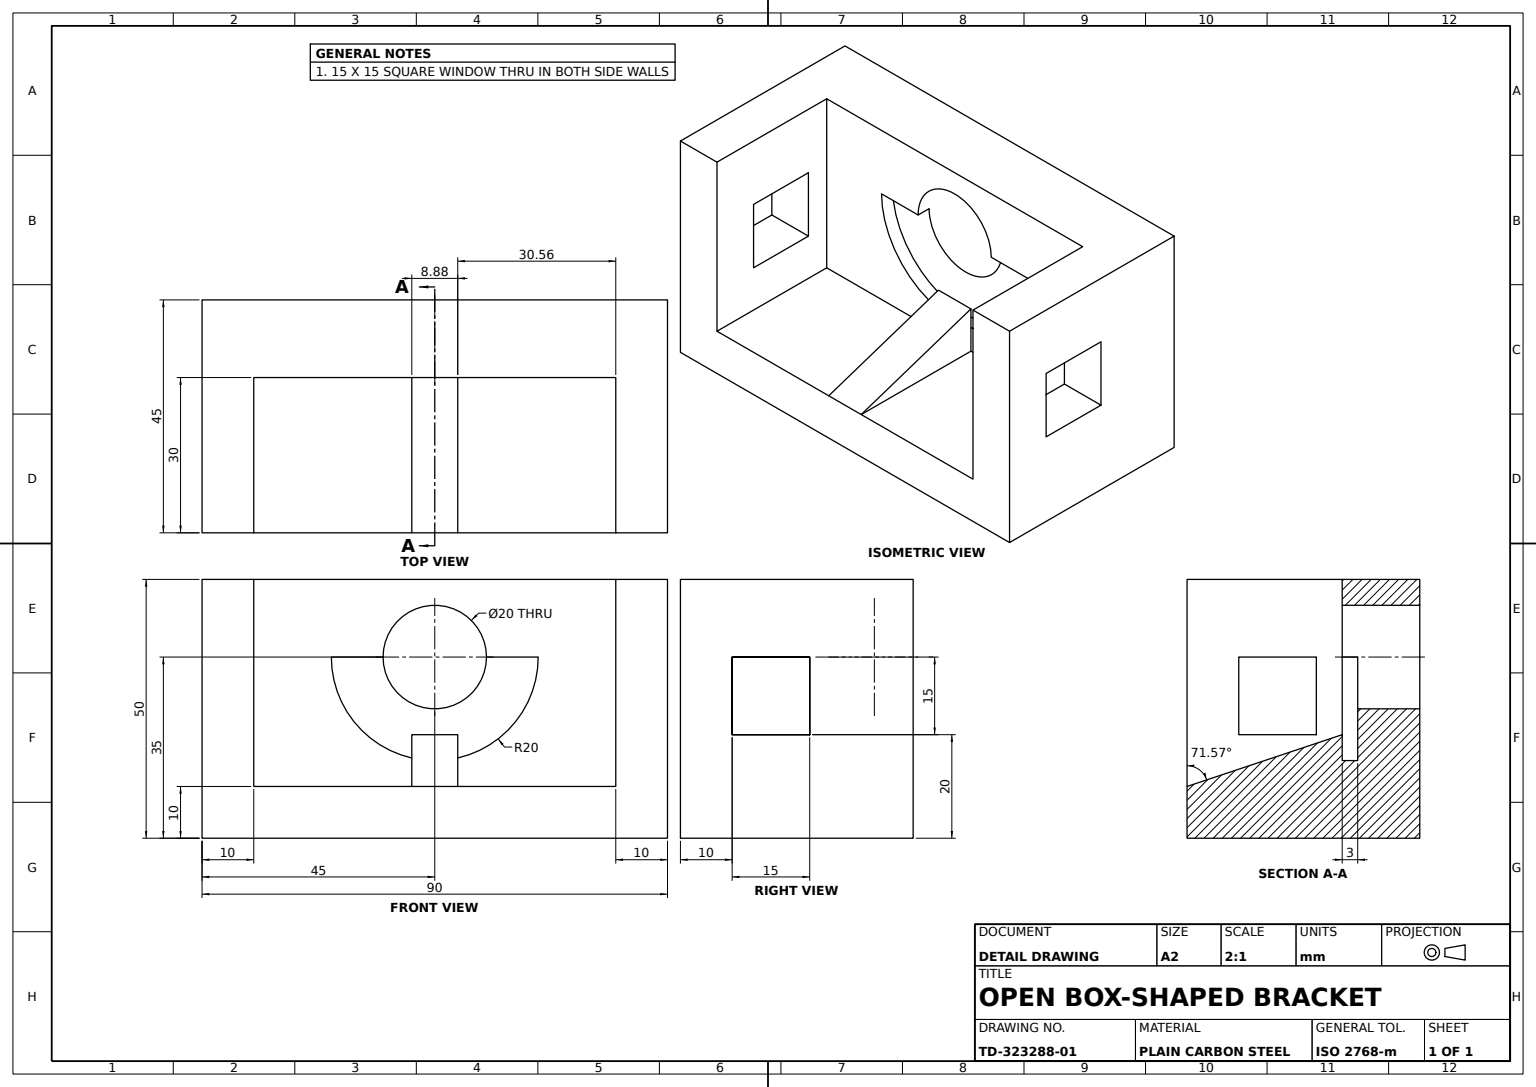
SolidWorks part; units mm, degrees
material "Plain Carbon Steel"
ref_plane "Front Plane" through (0, 0, 0) normal (0, 0, 1) x (1, 0, 0)
ref_plane "Top Plane" through (0, 0, 0) normal (0, 1, 0) x (1, 0, 0)
ref_plane "Right Plane" through (0, 0, 0) normal (1, 0, 0) x (0, 0, -1)
sketch "Block Profile Sketch 90x50" plane through (0, 0, 0) normal (0, 0, 1) x (1, 0, 0)
  line L1 (-45, 25) -> (45, 25)
  line L2 (-45, 25) -> (-45, -25)
  line L3 (-45, -25) -> (45, -25)
  line L4 (45, 25) -> (45, -25)
  line L5 (-45, 25) -> (45, -25) construction
  line L6 (-45, -25) -> (45, 25) construction
  point P0 (0, 0)
  dimension "D1" = 90
  dimension "D2" = 50
extrude "Base Block 90x50x45" add sketch "Block Profile Sketch 90x50" against normal blind 45
sketch "Pocket Sketch" plane through (0, 0, 0) normal (0, 0, 1) x (1, 0, 0)
  line L0 (45, -25) -> (45, 25) construction
  line L1 (45, 25) -> (-45, 25) construction
  line L2 (-35, 25) -> (-35, -15)
  line L3 (-35, -15) -> (35, -15)
  line L4 (35, -15) -> (35, 25)
  line L5 (35, 25) -> (-35, 25)
  dimension "D1" = 10
  dimension "D2" = 80
  dimension "D3" = 40
extrude "Inner Pocket 30 Deep" cut sketch "Pocket Sketch" against normal blind 30
sketch "Bore Sketch" plane through (0, 0, -30) normal (0, 0, 1) x (1, 0, 0)
  line L0 (0, 25) -> (0, 10) construction
  line L1 (35, 25) -> (-35, 25) construction
  circle A0 centre (0, 10) radius 10
  dimension "D1" = 20
  dimension "D2" = 15
extrude "Guide Bore Cut" cut sketch "Bore Sketch" against normal through all
sketch "Side Window Sketch" plane through (-45, 0, 0) normal (-1, 0, 0) x (0, 0, 1)
  line L0 (-45, -25) -> (-25, -25) construction
  line L1 (-45, -25) -> (0, -25) construction
  line L2 (-25, -25) -> (-25, -5) construction
  line L3 (-25, -5) -> (-25, 10)
  line L4 (-25, 10) -> (-10, 10)
  line L5 (-10, 10) -> (-10, -5)
  line L6 (-10, -5) -> (-25, -5)
  dimension "D1" = 15
  dimension "D2" = 15
  dimension "D3" = 20
  dimension "D4" = 20
extrude "Side Windows 15x15" cut sketch "Side Window Sketch" against normal through all
sketch "Rib Sketch" plane through (0, 0, -30) normal (0, 0, 1) x (1, 0, 0)
  line L0 (-35, -15) -> (35, -15) construction
  line L1 (4.4407, -5) -> (-4.4407, -5)
  line L2 (4.4407, -5) -> (4.4407, -15)
  line L3 (4.4407, -15) -> (-4.4407, -15)
  line L4 (-4.4407, -5) -> (-4.4407, -15)
  line L5 (4.4407, -5) -> (-4.4407, -15) construction
  line L6 (4.4407, -15) -> (-4.4407, -5) construction
  line L7 (-35, 25) -> (-35, -15) construction
  line L8 (35, 25) -> (-35, 25) construction
  point P0 (0, -10)
  dimension "D1" = 30.5593
  dimension "D2" = 35
  dimension "D3" = 30
extrude "Internal Rib" add sketch "Rib Sketch" along normal blind 30
sketch "Arc Groove Sketch" plane through (0, 0, -30) normal (0, 0, 1) x (1, 0, 0)
  line L0 (20, 10) -> (10, 10)
  line L1 (-10, 10) -> (-20, 10)
  arc A0 (-20, 10) -> (20, 10) centre (0, 10) ccw
  arc A1 (-10, 10) -> (10, 10) centre (0, 10) ccw
  dimension "D1" = 20
extrude "Arc Relief Groove 3 Deep" cut sketch "Arc Groove Sketch" against normal blind 3
sketch "Rib Trim Sketch" plane through (4.4407, 0, 0) normal (1, 0, 0) x (0, 0, -1)
  line L0 (30, -5) -> (0, -5)
  line L1 (0, -5) -> (0, -15)
  line L2 (0, -15) -> (30, -5)
extrude "Rib Trim Cut 10 Deep" cut sketch "Rib Trim Sketch" against normal blind 10
